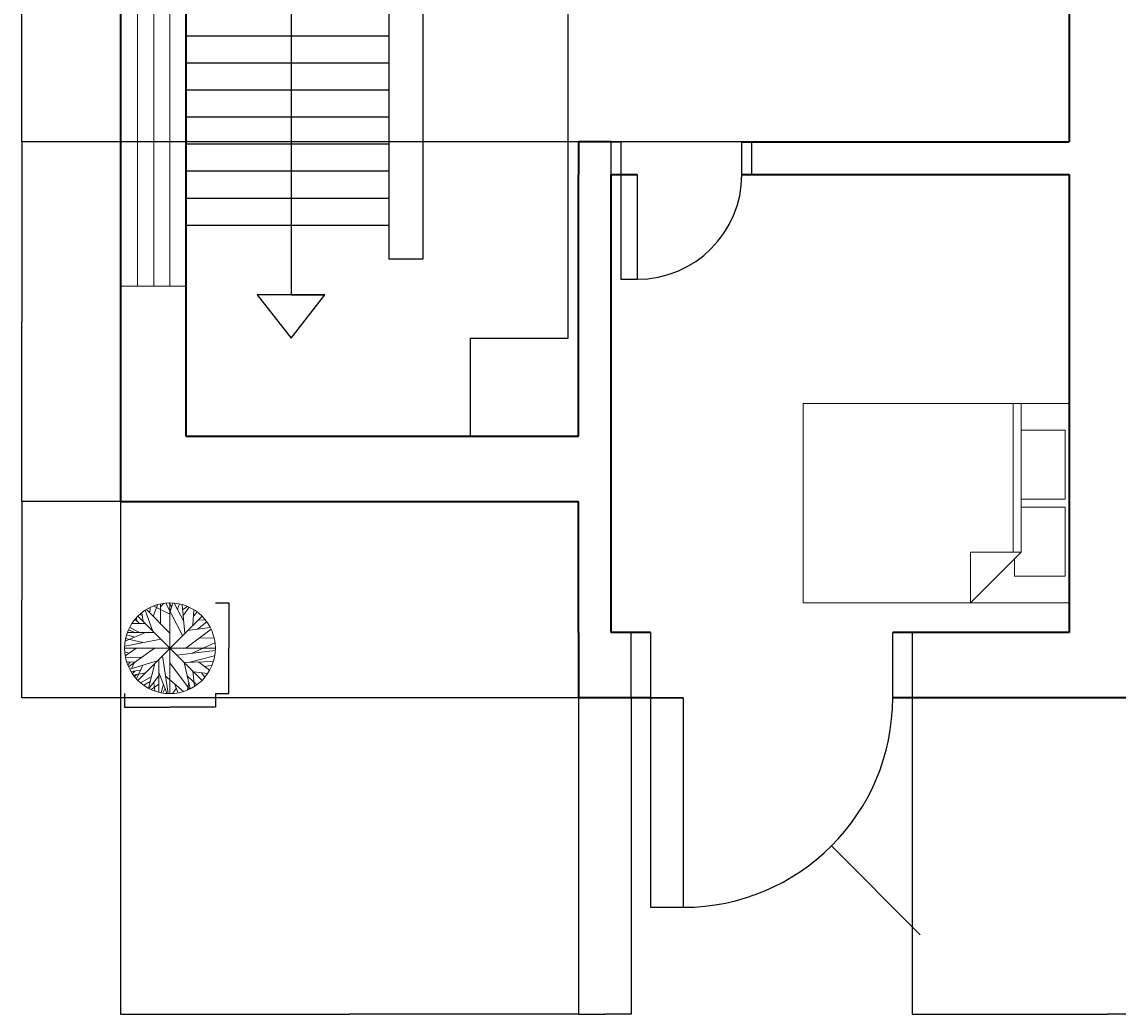
# Model space of a CAD drawing. Units: millimetres. Extents: x 726 to 37095, y -1634 to 13537.
# Tile 3 of 4: x 20550 to 28928, y -1634 to 5952. Entities that reach past the tile are written whole.
import ezdxf

# ---------------------------------------------------------------- set-up
doc = ezdxf.new("R2010")
doc.units = ezdxf.units.MM
for name, color, linetype, lineweight in [('A-ANNO-DIMS', 2, 'Continuous', 18), ('A-DOOR', 3, 'Continuous', 25), ('A-FLOR-STRS', 5, 'Continuous', 25), ('A-FURN', 8, 'Continuous', 18), ('A-GLAZ', 4, 'Continuous', 18), ('A-WALL', 7, 'Continuous', 35), ('L-PLNT', 94, 'Continuous', 18)]:
    doc.layers.add(name, color=color, linetype=linetype, lineweight=lineweight)
doc.styles.get("Standard").update_dxf_attribs({"font": 'arial.ttf'})
doc.dimstyles.get("Standard").update_dxf_attribs({"dimtxt": 0.18, "dimasz": 0.18, "dimexe": 0.18, "dimexo": 0.0625, "dimgap": 0.09, "dimtad": 0, "dimtih": 1, "dimtoh": 1, "dimdec": 4, "dimzin": 0, "dimdsep": 46, "dimtxsty": 'Standard', "dimcen": 0.09, "dimadec": 0, "dimazin": 0, "dimtfac": 1, "dimtdec": 4, "dimtofl": 0, "dimtmove": 0, "dimatfit": 3, "dimfxl": 1, "dimtolj": 1, "dimtzin": 0, "dimarcsym": 0})

# ---------------------------------------------------------------- blocks, each defined once
blk = doc.blocks.new('Window - Wood Frame 36 in. Wide plan')
for p, q in [((0, 6), (0, 0)), ((36, 6), (36, 0)), ((0, 4.5), (36, 4.5)), ((0, 3), (36, 3)), ((0, 1.5), (36, 1.5))]:
    blk.add_line(p, q)
blk = doc.blocks.new('Bed - Queen')
for p, q in [((0, -80.00003000000002), (0, 0)), ((0, 0), (59.99998999999999, 0)), ((59.99998999999999, 0), (59.99998999999999, -80.00003000000002)), ((7.99999, -1.200000000000017), (28.79998, -1.200000000000017)), ((7.99999, -14.4), (7.99999, -1.200000000000017)), ((28.79998, -1.200000000000017), (28.79998, -14.4)), ((31.19999, -1.200000000000017), (51.99999000000001, -1.200000000000017)), ((31.19999, -14.4), (31.19999, -1.200000000000017)), ((51.99999000000001, -1.200000000000017), (51.99999000000001, -16.4)), ((0, -14.4), (44.79999999999999, -14.4)), ((59.99998999999999, -29.60000000000001), (44.79999999999999, -14.4)), ((44.79999999999999, -14.4), (44.79999999999999, -29.60000000000001)), ((51.99999000000001, -16.4), (46.79936, -16.4)), ((44.79999999999999, -16.80000000000001), (0, -16.80000000000001)), ((44.79999999999999, -29.60000000000001), (59.99998999999999, -29.60000000000001)), ((59.99998999999999, -80.00003000000002), (0, -80.00003000000002))]:
    blk.add_line(p, q)
blk = doc.blocks.new('Tree - deciduous plan')
for p, q in [((-12.53879999999992, 54.94059999999979), (-7.961299999999937, 59.45459999999991)), ((-12.36270000000002, 32.14429999999993), (-12.53879999999992, 58.77760000000001)), ((-5.320499999999924, 59.68059999999979), (16.51049999999998, 16.79629999999986)), ((2.426000000000044, 54.94059999999979), (-1.447199999999952, 59.90559999999982)), ((0, 59.99959999999987), (0, -60.00000000000011)), ((0.4894000000000461, 48.62079999999991), (3.658400000000028, 59.68059999999979)), ((18.27110000000004, 35.52979999999991), (5.418999999999982, 59.68059999999979)), ((9.820299999999975, 51.55489999999986), (12.81330000000002, 58.55159999999989)), ((-40.17970000000002, 44.55799999999988), (-36.48249999999996, 43.20379999999988)), ((-37.01069999999993, 47.04079999999987), (-35.25, 35.52979999999991)), ((-32.60919999999999, 50.42639999999995), (-23.27819999999997, 23.56739999999991)), ((-31.20079999999996, 51.10349999999994), (-0.2148999999999432, 20.18179999999984)), ((-26.44719999999995, 46.58939999999984), (-26.27120000000002, 53.81159999999988)), ((-22.04579999999999, 42.07529999999986), (-16.58809999999994, 57.64859999999988)), ((-21.16559999999993, 55.84359999999981), (-0.0387999999999238, 45.00939999999991)), ((19.67950000000007, 19.50469999999984), (16.33440000000007, 57.64859999999988)), ((17.03870000000006, 51.10349999999994), (23.20060000000001, 55.16659999999991)), ((17.74290000000007, 43.65519999999992), (25.48940000000005, 54.26359999999988)), ((31.65129999999999, 50.87779999999987), (30.24290000000008, 30.56429999999989)), ((31.1232, 42.52669999999989), (35.87670000000003, 48.16929999999991)), ((-49.86270000000001, 32.82139999999993), (-32.78530000000001, 32.82139999999993)), ((-45.81339999999999, 38.23829999999987), (-40.53179999999997, 33.04709999999989)), ((-43.8768, 36.43259999999998), (-44.40499999999997, 40.26959999999997)), ((42, 41.99999999999988), (-42, -42.00000000000011)), ((42, -42.00000000000011), (-42, 41.99999999999988)), ((36.22879999999998, 25.14739999999995), (48.90489999999999, 35.07839999999987)), ((37.10910000000001, 37.10979999999995), (46.61609999999996, 37.56119999999987)), ((-32.25709999999992, 20.63329999999985), (-59.19370000000004, 9.347999999999843)), ((-57.08100000000001, 17.92479999999989), (-47.04579999999999, 14.7648999999999)), ((-56.02469999999994, 20.85899999999992), (-20.8134, 20.85899999999992)), ((-54.79229999999995, 24.47019999999986), (-47.75, 21.08469999999988)), ((-53.20780000000002, 27.4043999999999), (-40.17970000000002, 20.85899999999992)), ((54.36260000000004, 25.37309999999991), (20.91190000000006, 0.3197999999998728)), ((23.37670000000003, 23.34169999999994), (53.30629999999996, 27.4043999999999)), ((-59.72190000000001, 2.802499999999895), (-12.01059999999995, 12.05649999999991)), ((-58.66559999999992, 12.73359999999991), (-35.95429999999999, 7.542399999999929)), ((-54.61619999999993, -24.73350000000016), (-20.28530000000001, 0.0940999999999122)), ((29.36260000000004, -6.677100000000109), (59.46820000000002, 7.090999999999894)), ((38.51750000000004, 13.4106999999999), (58.23590000000002, 13.63639999999987)), ((-60, -1.137e-13), (60, -1.137e-13)), ((-59.72190000000001, -4.871400000000107), (-54.26409999999998, -6.677100000000109)), ((-45.2853, -0.1316000000001622), (-59.01769999999999, -10.06270000000006)), ((-58.48950000000002, -12.31970000000012), (-36.48249999999996, -11.64260000000013)), ((-10.07399999999995, -10.06270000000006), (-2.503600000000005, -59.71780000000013)), ((9.29219999999998, -9.159800000000132), (59.64430000000004, -2.84010000000012)), ((26.36969999999997, -18.41380000000015), (58.94010000000003, -9.836900000000128)), ((-57.08100000000001, -18.41380000000015), (-45.2853, -17.9624)), ((-52.67970000000002, -18.1880000000001), (-55.49659999999994, -22.02510000000007)), ((-53.20780000000002, -27.44200000000012), (-16.76409999999998, -16.60810000000015)), ((-47.2219, -19.31660000000011), (-50.21479999999996, -26.31350000000009)), ((-35.95429999999999, -22.4765000000001), (-44.05290000000002, -40.53290000000015)), ((-19.93309999999997, -20.21940000000018), (-28.55989999999997, -52.72100000000012)), ((-14.82749999999998, -15.02820000000008), (-14.65149999999994, -57.68650000000014)), ((-0.0387999999999238, -19.09090000000015), (25.8415, -53.84950000000015)), ((18.6232, -18.63940000000013), (26.72180000000003, -53.39810000000011)), ((18.79920000000004, -18.63940000000013), (57.35559999999998, -17.28530000000012)), ((38.16539999999998, -18.1880000000001), (52.42600000000004, -29.02190000000008)), ((45.91190000000006, -24.05640000000017), (55.59500000000003, -22.25080000000014)), ((-38.94719999999995, -29.02190000000008), (-51.44719999999995, -30.60180000000014)), ((-46.51769999999999, -30.15040000000011), (-49.51059999999995, -33.53600000000006)), ((-32.43309999999997, -32.40750000000014), (-48.10209999999995, -35.56740000000002)), ((-43.70079999999996, -34.66450000000009), (-46.69370000000003, -37.37300000000016)), ((-24.68669999999998, -37.8244000000002), (-38.77120000000002, -45.72410000000013)), ((-14.65149999999994, -36.24450000000013), (-27.67970000000003, -52.94670000000007)), ((-14.65149999999994, -32.18180000000007), (-3.912000000000034, -59.49220000000014)), ((-6.200799999999958, -36.24450000000013), (17.91899999999998, -57.00940000000014)), ((22.84850000000006, -36.47020000000009), (35.34850000000006, -48.43260000000009)), ((30.41899999999998, -30.15040000000011), (32.35559999999998, -50.01250000000016)), ((31.47530000000006, -31.27900000000011), (49.60910000000001, -33.3103000000001)), ((41.51049999999997, -32.6332000000001), (46.08799999999996, -38.05010000000016)), ((-26.27120000000002, -43.91850000000011), (-34.72190000000001, -48.65830000000006)), ((-14.65149999999994, -47.30410000000006), (-25.03879999999993, -54.30090000000006)), ((-21.51769999999999, -45.49840000000005), (-19.93309999999997, -56.1065000000001)), ((-8.48950000000002, -47.52980000000014), (-11.48249999999996, -58.58930000000009)), ((-6.376800000000002, -52.72100000000012), (-9.369799999999941, -58.81500000000006)), ((8.41190000000006, -53.17240000000004), (3.834400000000073, -59.49220000000014)), ((5.947099999999977, -46.62690000000009), (10.52459999999996, -58.58930000000009)), ((24.78520000000003, -44.82130000000006), (23.02459999999996, -54.97800000000006))]:
    blk.add_line(p, q)
blk.add_circle((0, -1.137e-13), 60)
blk = doc.blocks.new('DOOR-SWING-800')
for p, q in [((999.1999999999979, 1050), (874.1999999999979, 1050)), ((874.1999999999979, 250), (874.1999999999979, 1050)), ((999.1999999999979, 250), (999.1999999999979, 1050)), ((9.095e-13, 250), (74.199999999998, 250)), ((9.095e-13, 0), (9.095e-13, 250)), ((74.199999999998, 250), (74.199999999998, 0)), ((874.1999999999979, 250), (999.1999999999979, 250)), ((999.1999999999979, 250), (1073.400000000002, 250)), ((999.1999999999979, 0), (999.1999999999979, 250)), ((1073.400000000002, 250), (1073.400000000002, 0)), ((74.199999999998, 0), (9.095e-13, 0)), ((1073.400000000002, 0), (999.1999999999979, 0))]:
    blk.add_line(p, q)
blk.add_arc((874.1999999999979, 250), 800, 90, 180)
blk = doc.blocks.new('DOOR-ENTRY-1601')
for p, q in [((0, 1600.959499914892), (0, 2101.259343638296)), ((0, 2101.259343638296), (148.488993617113, 2101.259343638296)), ((148.488993617113, 2101.259343638296), (148.488993617113, 1600.959499914892)), ((1999.598415393706, 1600.959499914892), (1999.598415393706, 2101.259343638296)), ((1999.598415393706, 2101.259343638296), (2148.087409010808, 2101.259343638296)), ((2148.087409010808, 2101.259343638296), (2148.087409010808, 1600.959499914892)), ((148.488993617113, 1600.959499914892), (0, 1600.959499914892)), ((148.488993617113, 1600.959499914892), (148.488993617113, -1.137e-13)), ((398.6389154788158, 1600.959499914892), (148.488993617113, 1600.959499914892)), ((148.488993617113, 1600.959499914892), (398.6389154788158, 1600.959499914892)), ((398.6389154788158, 1600.959499914892), (398.6389154788158, -1.137e-13)), ((2148.087409010808, 1600.959499914892), (1999.598415393706, 1600.959499914892)), ((148.488993617113, -1.137e-13), (398.6389154788158, -1.137e-13))]:
    blk.add_line(p, q)
blk.add_arc((398.6389154788158, 1600.959499914892), 1600.959499914892, 270, 0)
blk = doc.blocks.new('STAIR-QUARTER-TURN')
for p, q in [((1551.94660387568, 5000.000000000002), (1551.94660387568, 3551.516503049365)), ((1758.872817725773, 5000.000000000002), (1758.872817725773, 3551.516503049365)), ((1965.799031575862, 5000.000000000002), (1965.799031575862, 3551.516503049365)), ((2172.725245425954, 5000.000000000002), (2172.725245425954, 3551.516503049365)), ((2172.725245425954, 4193.579423830473), (803.743340616409, 4193.579423830471)), ((803.743340616409, 4193.579423830471), (803.743340616409, 330.5564002077117)), ((2172.725245425954, 3551.516503049366), (0, 3551.516503049365)), ((1551.94660387568, 3551.516503049365), (1551.94660387568, 3344.590289199272)), ((2172.725245425954, 3551.516503049365), (2172.725245425954, 3292.858735736751)), ((1551.94660387568, 3344.590289199272), (0, 3344.590289199273)), ((1551.94660387568, 3344.590289199272), (1551.94660387568, 861.4757229981805)), ((2172.725245425954, 3292.858735736751), (1810.604371188295, 3292.858735736751)), ((1810.604371188295, 3292.85873573675), (1810.604371188295, 602.8179556856148)), ((1551.94660387568, 3137.664075349182), (0, 3137.664075349182)), ((1551.94660387568, 2930.73786149909), (0, 2930.737861499091)), ((1551.94660387568, 2723.811647649), (0, 2723.811647649001)), ((1551.94660387568, 2516.885433798908), (0, 2516.885433798909)), ((1551.94660387568, 2309.959219948817), (0, 2309.959219948818)), ((1551.94660387568, 2103.033006098726), (0, 2103.033006098727)), ((1551.94660387568, 1896.106792248635), (0, 1896.106792248635)), ((1551.94660387568, 1689.180578398543), (0, 1689.180578398544)), ((1551.94660387568, 1482.254364548453), (0, 1482.254364548454)), ((1551.94660387568, 1275.328150698362), (0, 1275.328150698363)), ((1551.94660387568, 1068.40193684827), (0, 1068.401936848271)), ((1551.94660387568, 861.4757229981795), (0, 861.4757229981805)), ((1551.94660387568, 861.4757229981805), (1551.946603875687, 602.8179556856074)), ((1810.604371188295, 602.8179556856148), (1551.946603875687, 602.8179556855675)), ((803.743340616409, 330.5564002077117), (545.0855733037969, 330.5564002077117)), ((545.0855733037969, 330.5564002077117), (803.743340616409, 4.547e-13)), ((803.743340616409, 330.5564002077117), (1062.401107929021, 330.5564002077108)), ((803.743340616409, 4.547e-13), (1062.401107929021, 330.5564002077117))]:
    blk.add_line(p, q)
blk = doc.blocks.new('*D35')
at = {"layer": 'A-ANNO-DIMS', "color": 0, "lineweight": -2, "transparency": 16777216}
for p, q in [((23976.18779894455, 8533.885868122888), (24726.30529894457, 8533.885868122888)), ((24726.12529894457, 8533.705868122888), (24726.12529894457, 6034.068937699966)), ((24726.12529894457, 3534.065868122886), (24726.12529894457, 6033.702798545806)), ((23976.18779894455, 3533.885868122886), (24726.30529894458, 3533.885868122886))]:
    blk.add_line(p, q, dxfattribs=at)
at = {"layer": 'A-ANNO-DIMS', "color": 0, "transparency": 16777216}
for points in [[(24726.09529894457, 8533.705868122888), (24726.15529894457, 8533.705868122888), (24726.12529894457, 8533.885868122888)], [(24726.09529894458, 3534.065868122886), (24726.15529894457, 3534.065868122886), (24726.12529894457, 3533.885868122886)]]:
    blk.add_solid(points, dxfattribs=at)
at = {"layer": 'Defpoints', "color": 0, "transparency": 16777216}
for p in [(23976.12529894455, 8533.885868122888), (24726.12529894457, 8533.885868122888), (23976.12529894455, 3533.885868122886)]:
    blk.add_point(p, dxfattribs=at)
at = {"layer": 'A-ANNO-DIMS', "color": 0, "transparency": 16777216, "insert": (24726.12529894457, 6033.885868122878), "char_height": 0.18, "attachment_point": 5}
blk.add_mtext('\\A1;STAIR 5000 TYP.', dxfattribs=at)
blk = doc.blocks.new('*D36')
at = {"layer": 'A-ANNO-DIMS', "color": 0, "lineweight": -2, "transparency": 16777216}
for p, q in [((21803.40005351859, 3533.823368122884), (21803.40005351859, 2783.705868122883)), ((23976.12529894455, 3533.823368122884), (23976.12529894455, 2783.705868122883)), ((21803.58005351859, 2783.885868122883), (22889.09320147031, 2783.885868122883)), ((23975.94529894455, 2783.885868122883), (22890.43215099283, 2783.885868122883))]:
    blk.add_line(p, q, dxfattribs=at)
at = {"layer": 'A-ANNO-DIMS', "color": 0, "transparency": 16777216}
for points in [[(21803.58005351859, 2783.915868122884), (21803.58005351859, 2783.855868122883), (21803.40005351859, 2783.885868122883)], [(23975.94529894455, 2783.915868122884), (23975.94529894455, 2783.855868122883), (23976.12529894455, 2783.885868122883)]]:
    blk.add_solid(points, dxfattribs=at)
at = {"layer": 'Defpoints', "color": 0, "transparency": 16777216}
for p in [(21803.40005351859, 3533.885868122883), (23976.12529894455, 3533.885868122883), (23976.12529894455, 2783.885868122883)]:
    blk.add_point(p, dxfattribs=at)
at = {"layer": 'A-ANNO-DIMS', "color": 0, "transparency": 16777216, "insert": (22889.76267623157, 2783.885868122883), "char_height": 0.18, "attachment_point": 5}
blk.add_mtext('\\A1;2173 TYP.', dxfattribs=at)
blk = doc.blocks.new('*D41')
at = {"layer": 'A-ANNO-DIMS', "color": 0, "lineweight": -2, "transparency": 16777216}
for p, q in [((21334.8865153471, 815.9126766530406), (21334.8865153471, 711.7131389074812)), ((22028.76676698416, 815.9126766530406), (22028.76676698416, 711.7131389074812)), ((21335.06651534709, 711.8931389074812), (21680.85610228432, 711.8931389074812)), ((22028.58676698416, 711.8931389074812), (21682.79718004694, 711.8931389074812))]:
    blk.add_line(p, q, dxfattribs=at)
at = {"layer": 'A-ANNO-DIMS', "color": 0, "transparency": 16777216}
for points in [[(21335.06651534709, 711.9231389074812), (21335.06651534709, 711.8631389074812), (21334.8865153471, 711.8931389074812)], [(22028.58676698416, 711.9231389074812), (22028.58676698416, 711.8631389074812), (22028.76676698416, 711.8931389074812)]]:
    blk.add_solid(points, dxfattribs=at)
at = {"layer": 'Defpoints', "color": 0, "transparency": 16777216}
for p in [(21334.8865153471, 815.9751766530406), (22028.76676698416, 815.9751766530406), (22028.76676698416, 711.8931389074812)]:
    blk.add_point(p, dxfattribs=at)
at = {"layer": 'A-ANNO-DIMS', "color": 0, "transparency": 16777216, "insert": (21681.82664116563, 711.8931389074812), "char_height": 0.18, "attachment_point": 5}
blk.add_mtext('\\A1;TREE 694 TYP.', dxfattribs=at)
blk = doc.blocks.new('*D42')
at = {"layer": 'A-ANNO-DIMS', "color": 0, "lineweight": -2, "transparency": 16777216}
for p, q in [((22028.82926698417, 1509.855428290102), (22133.02880472974, 1509.855428290102)), ((22132.84880472974, 1509.675428290102), (22132.84880472974, 1163.097205609362)), ((22132.84880472974, 816.155176653041), (22132.84880472974, 1162.733399333782)), ((22028.82926698417, 815.9751766530412), (22133.02880472974, 815.9751766530412))]:
    blk.add_line(p, q, dxfattribs=at)
at = {"layer": 'A-ANNO-DIMS', "color": 0, "transparency": 16777216}
for points in [[(22132.81880472974, 1509.675428290102), (22132.87880472973, 1509.675428290102), (22132.84880472974, 1509.855428290102)], [(22132.81880472974, 816.155176653041), (22132.87880472973, 816.155176653041), (22132.84880472974, 815.9751766530412)]]:
    blk.add_solid(points, dxfattribs=at)
at = {"layer": 'Defpoints', "color": 0, "transparency": 16777216}
for p in [(22028.76676698417, 1509.855428290102), (22132.84880472974, 1509.855428290102), (22028.76676698417, 815.9751766530412)]:
    blk.add_point(p, dxfattribs=at)
at = {"layer": 'A-ANNO-DIMS', "color": 0, "transparency": 16777216, "insert": (22132.84880472973, 1162.915302471565), "char_height": 0.18, "attachment_point": 5}
blk.add_mtext('\\A1;694 TYP.', dxfattribs=at)
blk = doc.blocks.new('*D65')
at = {"layer": 'A-ANNO-DIMS', "color": 0, "lineweight": -2, "transparency": 16777216}
for p, q in [((21303.400054, 2283.823368), (21303.400054, -1633.776092999999)), ((24803.400054, 2283.823368), (24803.400054, -1633.776092999999)), ((21303.580054, -1633.596093), (23053.04165018009, -1633.596093)), ((24803.220054, -1633.596093), (23053.75845781992, -1633.596093))]:
    blk.add_line(p, q, dxfattribs=at)
at = {"layer": 'A-ANNO-DIMS', "color": 0, "transparency": 16777216}
for points in [[(21303.580054, -1633.566093), (21303.580054, -1633.626093), (21303.400054, -1633.596093)], [(24803.220054, -1633.566093), (24803.220054, -1633.626093), (24803.400054, -1633.596093)]]:
    blk.add_solid(points, dxfattribs=at)
at = {"layer": 'Defpoints', "color": 0, "transparency": 16777216}
for p in [(21303.400054, 2283.885868), (24803.400054, 2283.885868), (24803.400054, -1633.596093)]:
    blk.add_point(p, dxfattribs=at)
at = {"layer": 'A-ANNO-DIMS', "color": 0, "transparency": 16777216, "insert": (23053.400054, -1633.596093), "char_height": 0.18, "attachment_point": 5}
blk.add_mtext('\\A1;3500', dxfattribs=at)
blk = doc.blocks.new('*D67')
at = {"layer": 'A-ANNO-DIMS', "color": 0, "lineweight": -2, "transparency": 16777216}
for p, q in [((21303.33755400001, 2283.885868000001), (20550.47005400002, 2283.885868000001)), ((20550.65005400002, 2283.705868000001), (20550.65005400002, 1534.06777113779)), ((20550.65005400002, 784.0658679999997), (20550.65005400002, 1533.70396486221)), ((24803.33755400002, 783.8858680000003), (20550.47005400002, 783.8858679999997))]:
    blk.add_line(p, q, dxfattribs=at)
at = {"layer": 'A-ANNO-DIMS', "color": 0, "transparency": 16777216}
for points in [[(20550.62005400002, 2283.705868000001), (20550.68005400002, 2283.705868000001), (20550.65005400002, 2283.885868000001)], [(20550.62005400002, 784.0658679999997), (20550.68005400002, 784.0658679999997), (20550.65005400002, 783.8858679999997)]]:
    blk.add_solid(points, dxfattribs=at)
at = {"layer": 'Defpoints', "color": 0, "transparency": 16777216}
for p in [(21303.40005400001, 2283.885868000001), (20550.65005400002, 783.8858679999997), (24803.40005400002, 783.8858680000003)]:
    blk.add_point(p, dxfattribs=at)
at = {"layer": 'A-ANNO-DIMS', "color": 0, "transparency": 16777216, "insert": (20550.65005400001, 1533.885867999994), "char_height": 0.18, "attachment_point": 5}
blk.add_mtext('\\A1;1500', dxfattribs=at)
blk = doc.blocks.new('*D68')
at = {"layer": 'A-ANNO-DIMS', "color": 0, "lineweight": -2, "transparency": 16777216}
for p, q in [((24803.33755400002, 5033.885868000002), (20550.47005400002, 5033.885868000002)), ((20550.65005400002, 5033.705868000001), (20550.65005400002, 3659.067771137791)), ((20550.65005400002, 2284.065868), (20550.65005400002, 3658.703964862211)), ((24803.33755400002, 2283.885868000001), (20550.47005400002, 2283.885868))]:
    blk.add_line(p, q, dxfattribs=at)
at = {"layer": 'A-ANNO-DIMS', "color": 0, "transparency": 16777216}
for points in [[(20550.62005400002, 5033.705868000001), (20550.68005400002, 5033.705868000001), (20550.65005400002, 5033.885868000002)], [(20550.62005400002, 2284.065868), (20550.68005400002, 2284.065868), (20550.65005400002, 2283.885868)]]:
    blk.add_solid(points, dxfattribs=at)
at = {"layer": 'Defpoints', "color": 0, "transparency": 16777216}
for p in [(20550.65005400002, 5033.885868000002), (24803.40005400002, 5033.885868000002), (24803.40005400002, 2283.885868000001)]:
    blk.add_point(p, dxfattribs=at)
at = {"layer": 'A-ANNO-DIMS', "color": 0, "transparency": 16777216, "insert": (20550.65005400001, 3658.885867999994), "char_height": 0.18, "attachment_point": 5}
blk.add_mtext('\\A1;2750', dxfattribs=at)
blk = doc.blocks.new('*D73')
at = {"layer": 'A-ANNO-DIMS', "color": 0, "lineweight": -2, "transparency": 16777216}
for p, q in [((28553.33755400002, 8533.885868000005), (20550.47005400001, 8533.885868000005)), ((20550.65005400001, 8533.705868000003), (20550.65005400002, 6784.067832529334)), ((20550.65005400002, 5034.065868000002), (20550.65005400002, 6783.70390347067)), ((28553.33755400002, 5033.885868000002), (20550.47005400002, 5033.885868000002))]:
    blk.add_line(p, q, dxfattribs=at)
at = {"layer": 'A-ANNO-DIMS', "color": 0, "transparency": 16777216}
for points in [[(20550.62005400001, 8533.705868000003), (20550.68005400001, 8533.705868000003), (20550.65005400001, 8533.885868000005)], [(20550.62005400002, 5034.065868000002), (20550.68005400002, 5034.065868000002), (20550.65005400002, 5033.885868000002)]]:
    blk.add_solid(points, dxfattribs=at)
at = {"layer": 'Defpoints', "color": 0, "transparency": 16777216}
for p in [(20550.65005400001, 8533.885868000005), (28553.40005400002, 8533.885868000005), (28553.40005400002, 5033.885868000002)]:
    blk.add_point(p, dxfattribs=at)
at = {"layer": 'A-ANNO-DIMS', "color": 0, "transparency": 16777216, "insert": (20550.65005400001, 6783.885867999995), "char_height": 0.18, "attachment_point": 5}
blk.add_mtext('\\A1;3500', dxfattribs=at)
blk = doc.blocks.new('*D82')
at = {"layer": 'A-ANNO-DIMS', "color": 0, "lineweight": -2, "transparency": 16777216}
for p, q in [((24803.400054, 783.823368), (24803.400054, -1633.776092999999)), ((25206.416494, 783.523524), (25206.416494, -1633.776093)), ((24803.580054, -1633.596093), (25004.61580469577, -1633.596093)), ((25206.236494, -1633.596093), (25005.20074330423, -1633.596093))]:
    blk.add_line(p, q, dxfattribs=at)
at = {"layer": 'A-ANNO-DIMS', "color": 0, "transparency": 16777216}
for points in [[(24803.580054, -1633.566093), (24803.580054, -1633.626093), (24803.400054, -1633.596093)], [(25206.236494, -1633.566093), (25206.236494, -1633.626093), (25206.416494, -1633.596093)]]:
    blk.add_solid(points, dxfattribs=at)
at = {"layer": 'Defpoints', "color": 0, "transparency": 16777216}
for p in [(24803.400054, 783.8858679999998), (25206.416494, 783.586024), (25206.416494, -1633.596093)]:
    blk.add_point(p, dxfattribs=at)
at = {"layer": 'A-ANNO-DIMS', "color": 0, "transparency": 16777216, "insert": (25004.908274, -1633.596093), "char_height": 0.18, "attachment_point": 5}
blk.add_mtext('\\A1;403', dxfattribs=at)
blk = doc.blocks.new('*D83')
at = {"layer": 'A-ANNO-DIMS', "color": 0, "lineweight": -2, "transparency": 16777216}
for p, q in [((27354.503903, 783.523524), (27354.503903, -1633.776093)), ((30340.425495, 783.823368), (30340.425495, -1633.776092999999)), ((27354.683903, -1633.596093), (28847.10445343383, -1633.596093)), ((30340.245495, -1633.596093), (28847.82494456617, -1633.596093))]:
    blk.add_line(p, q, dxfattribs=at)
at = {"layer": 'A-ANNO-DIMS', "color": 0, "transparency": 16777216}
for points in [[(27354.683903, -1633.566093), (27354.683903, -1633.626093), (27354.503903, -1633.596093)], [(30340.245495, -1633.566093), (30340.245495, -1633.626093), (30340.425495, -1633.596093)]]:
    blk.add_solid(points, dxfattribs=at)
at = {"layer": 'Defpoints', "color": 0, "transparency": 16777216}
for p in [(27354.503903, 783.586024), (30340.425495, 783.8858679999998), (30340.425495, -1633.596093)]:
    blk.add_point(p, dxfattribs=at)
at = {"layer": 'A-ANNO-DIMS', "color": 0, "transparency": 16777216, "insert": (28847.464699, -1633.596093), "char_height": 0.18, "attachment_point": 5}
blk.add_mtext('\\A1;2986', dxfattribs=at)
blk = doc.blocks.new('*D88')
at = {"layer": 'A-ANNO-DIMS', "color": 0, "lineweight": -2, "transparency": 16777216}
for p, q in [((25604.96541, 783.5860240000056), (25605.14541, 783.5860240000038)), ((25605.05541, 783.4960240000037), (25605.05541, 783.6760240000021)), ((27416.33477211299, -1027.692432512991), (26737.23229025243, -348.5902901887966)), ((27416.51477211299, -1027.692432512991), (27416.33477211299, -1027.692432512991))]:
    blk.add_line(p, q, dxfattribs=at)
at = {"layer": 'A-ANNO-DIMS', "color": 0, "transparency": 16777216}
blk.add_solid([(26737.25350345057, -348.5690769800604), (26737.2110770543, -348.6115033975348), (26737.105011, -348.4630109999998)], dxfattribs=at)
at = {"layer": 'Defpoints', "color": 0, "transparency": 16777216}
for p in [(25605.05541, 783.5860240000038), (26737.105011, -348.4630109999998)]:
    blk.add_point(p, dxfattribs=at)
at = {"layer": 'A-ANNO-DIMS', "color": 0, "transparency": 16777216, "insert": (27416.94230280876, -1027.692432512989), "char_height": 0.18, "attachment_point": 5}
blk.add_mtext('\\A1;R1601', dxfattribs=at)

msp = doc.modelspace()

# ---------------------------------------------------------------- linework, layer by layer
at = {"layer": 'A-DOOR'}
for p, q in [((25053.40005351859, 5033.885868122886), (25127.60005351859, 5033.885868122885)), ((25053.40005351859, 5033.885868122886), (25127.60005351859, 5033.885868122886)), ((26052.60005351859, 5033.885868122884), (26126.80005351859, 5033.885868122882)), ((26052.60005351859, 5033.885868122886), (26126.80005351859, 5033.885868122886)), ((26052.60005351859, 5033.885868122887), (26126.80005351859, 5033.885868122889))]:
    msp.add_line(p, q, dxfattribs=at)
at = {"layer": 'A-FLOR-STRS'}
msp.add_line((22865.80116144761, 3864.442268330595), (22607.143394135, 3864.442268330595), dxfattribs=at)
at = {"layer": 'A-WALL'}
for p, q in [((21303.40005351859, 12783.88586812288), (21303.40005351859, 2283.885868122887)), ((21803.40005351859, 8533.885868122883), (21803.40005351859, 2783.885868122886)), ((28553.40005351859, 8533.885868122887), (28553.40005351859, 5033.885868122885)), ((25053.40005351859, 5033.885868122886), (24803.40005351858, 5033.885868122886)), ((24803.40005351858, 5033.885868122886), (24803.40005351859, 4783.885868122886)), ((26052.60005351859, 5033.885868122885), (28553.40005351859, 5033.885868122885)), ((24803.40005351859, 2783.885868122886), (24803.40005351859, 4783.885868122886)), ((25053.40005351859, 1283.885868122886), (25053.40005351859, 4783.885868122886)), ((25053.40005351859, 4783.885868122886), (25252.60005351859, 4783.885868122886)), ((26052.60005351859, 4783.885868122886), (28553.40005351859, 4783.885868122885)), ((28553.40005351859, 4783.885868122885), (28553.40005351859, 1283.885868122886)), ((21803.40005351859, 2783.885868122886), (24803.40005351859, 2783.885868122886)), ((21303.40005351859, 2283.885868122886), (24803.40005351859, 2283.885868122887)), ((24803.40005351859, 1283.885868122886), (24803.40005351859, 2283.885868122887)), ((24803.40005351859, 1283.885868122886), (24803.40005351858, 1033.885868122886)), ((25354.90548771432, 1283.885868122886), (25053.40005351859, 1283.885868122886)), ((28553.40005351859, 1283.885868122886), (27206.01490949092, 1283.885868122886)), ((24803.40005351859, 1033.885868122886), (24803.40005351858, 783.8858681228855)), ((25053.40005351859, 783.8858681228857), (24803.40005351858, 783.8858681228855)), ((25354.90548771432, 783.8858681228859), (25053.40005351859, 783.8858681228857)), ((28553.40005351859, 783.8858681228857), (27206.01490949092, 783.8858681228859)), ((29053.4000535186, 783.8858681228855), (28553.40005351859, 783.8858681228857))]:
    msp.add_line(p, q, dxfattribs=at)

# ---------------------------------------------------------------- block references
at = {"layer": 'A-DOOR', "rotation": 180}
msp.add_blockref('DOOR-SWING-800', (26126.80005351859, 5033.885868122888), dxfattribs=at)
at = {"layer": 'A-DOOR'}
msp.add_blockref('DOOR-ENTRY-1601', (25206.41649409721, -817.3734755154034), dxfattribs=at)
at = {"layer": 'A-FLOR-STRS'}
msp.add_blockref('STAIR-QUARTER-TURN', (21803.40005351859, 3533.885868122883), dxfattribs=at)
at = {"layer": 'A-FURN', "xscale": 25.4, "yscale": 25.4, "zscale": 25.4, "rotation": 270}
msp.add_blockref('Bed - Queen', (28553.40005351859, 3034.61281299441), dxfattribs=at)
at = {"layer": 'A-GLAZ', "xscale": 81.8978551733564, "yscale": 81.8978551733564, "zscale": 81.8978551733564, "rotation": 270}
msp.add_blockref('Window - Wood Frame 36 in. Wide plan', (21312.01292247845, 6878.476157322156), dxfattribs=at)
at = {"layer": 'L-PLNT', "xscale": 5.782335430308843, "yscale": 5.782335430308843, "zscale": 5.782335430308843}
msp.add_blockref('Tree - deciduous plan', (21681.82664116563, 1162.915302471572), dxfattribs=at)

# ---------------------------------------------------------------- dimensions: what is measured, and where the dimension line sits
at = {"layer": 'A-ANNO-DIMS'}
for base, p1, p2, picture, middle in [((20550.65005400001, 8533.885868000005), (28553.400054, 5033.885868), (28553.400054, 8533.885868), '*D73', (20550.65005400001, 6783.885867999995)), ((20550.65005400002, 5033.885868000002), (24803.400054, 2283.885868), (24803.400054, 5033.885868), '*D68', (20550.65005400001, 3658.885867999994)), ((20550.65005400002, 783.8858679999997), (21303.400054, 2283.885868), (24803.400054, 783.8858679999998), '*D67', (20550.65005400001, 1533.885867999994))]:
    dim = msp.add_linear_dim(base=base, p1=p1, p2=p2, angle=90, dimstyle='Standard', override={"dimdec": 0, "dimlfac": 1, "dimrnd": 0, "dimzin": 0, "dimdsep": 46, "dimlunit": 2}, dxfattribs=at)
    dim.commit()
    dim.dimension.update_dxf_attribs({"geometry": picture, "text_midpoint": middle})
for base, p1, p2, text, picture, middle in [((24726.12529894457, 8533.885868122888), (23976.12529894455, 3533.885868122883), (23976.12529894455, 8533.885868122885), 'STAIR <> TYP.', '*D35', (24726.12529894457, 6033.885868122878)), ((22132.84880472974, 1509.855428290102), (22028.76676698416, 815.9751766530406), (22028.76676698416, 1509.855428290102), '<> TYP.', '*D42', (22132.84880472973, 1162.915302471565))]:
    dim = msp.add_linear_dim(base=base, p1=p1, p2=p2, angle=90, text=text, dimstyle='Standard', override={"dimdec": 0, "dimlfac": 1, "dimrnd": 0, "dimzin": 0, "dimdsep": 46, "dimlunit": 2}, dxfattribs=at)
    dim.commit()
    dim.dimension.update_dxf_attribs({"geometry": picture, "text_midpoint": middle})
for base, p1, p2, text, picture, middle in [((23976.12529894455, 2783.885868122883), (21803.40005351859, 3533.885868122883), (23976.12529894455, 3533.885868122883), '<> TYP.', '*D36', (22889.76267623157, 2783.885868122883)), ((22028.76676698416, 711.8931389074812), (21334.8865153471, 815.9751766530406), (22028.76676698416, 815.9751766530406), 'TREE <> TYP.', '*D41', (21681.82664116563, 711.8931389074812))]:
    dim = msp.add_linear_dim(base=base, p1=p1, p2=p2, text=text, dimstyle='Standard', override={"dimdec": 0, "dimlfac": 1, "dimrnd": 0, "dimzin": 0, "dimdsep": 46, "dimlunit": 2}, dxfattribs=at)
    dim.commit()
    dim.dimension.update_dxf_attribs({"geometry": picture, "text_midpoint": middle})
for base, p1, p2, picture, middle in [((24803.400054, -1633.596093), (21303.400054, 2283.885868), (24803.400054, 2283.885868), '*D65', (23053.400054, -1633.596093)), ((25206.416494, -1633.596093), (24803.400054, 783.8858679999998), (25206.416494, 783.586024), '*D82', (25004.908274, -1633.596093)), ((30340.425495, -1633.596093), (27354.503903, 783.586024), (30340.425495, 783.8858679999998), '*D83', (28847.464699, -1633.596093))]:
    dim = msp.add_linear_dim(base=base, p1=p1, p2=p2, dimstyle='Standard', override={"dimdec": 0, "dimlfac": 1, "dimrnd": 0, "dimzin": 0, "dimdsep": 46, "dimlunit": 2}, dxfattribs=at)
    dim.commit()
    dim.dimension.update_dxf_attribs({"geometry": picture, "text_midpoint": middle})
dim = msp.add_radius_dim(center=(25605.05541, 783.5860240000038), mpoint=(26737.105011, -348.4630109999998), dimstyle='Standard', override={"dimdec": 0, "dimlfac": 1, "dimrnd": 0, "dimzin": 0, "dimdsep": 46, "dimlunit": 2}, dxfattribs=at)
dim.commit()
dim.dimension.update_dxf_attribs({"geometry": '*D88', "text_midpoint": (27416.94230280876, -1027.692432512989), "dimtype": 164})

doc.saveas('drawing.dxf')
